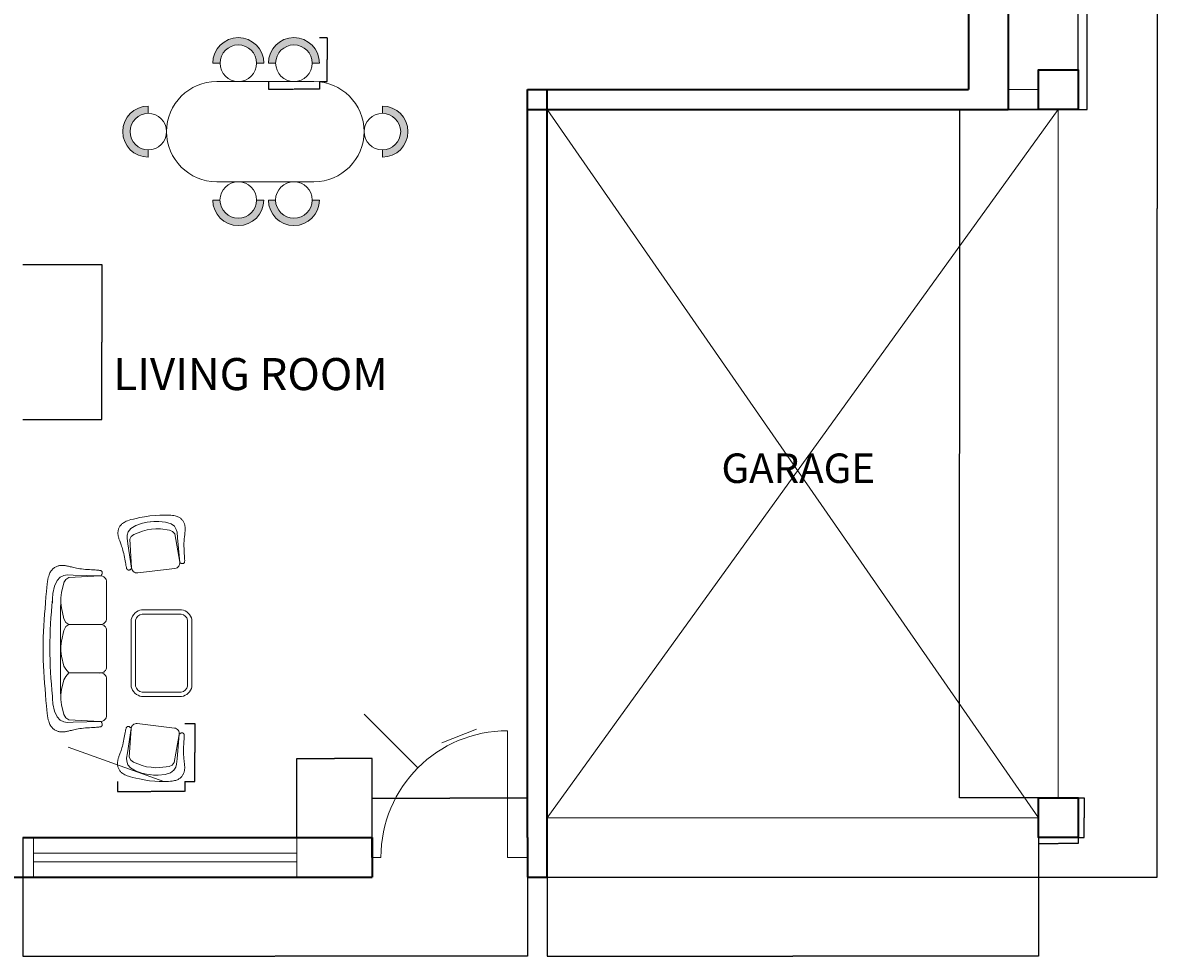
# Model space of a CAD drawing. Units: millimetres. Extents: x 2511 to 24632, y 2213 to 12972.
# Tile 2 of 5: x 6023 to 12605, y 2213 to 7630. Entities that reach past the tile are written whole.
import ezdxf

# ---------------------------------------------------------------- set-up
doc = ezdxf.new("R2010")
doc.units = ezdxf.units.MM
for name, color, linetype, lineweight in [('A-ANNO-DIMS', 2, 'Continuous', 18), ('A-AREA-IDEN', 7, 'Continuous', 20), ('A-COLS', 7, 'Continuous', 35), ('A-FLOR-GARG', 7, 'Continuous', 18), ('A-WALL', 7, 'Continuous', 35), ('doors', 50, 'Continuous', 18), ('Imaginery', 30, 'Continuous', 13), ('windows', 70, 'Continuous', 18)]:
    doc.layers.add(name, color=color, linetype=linetype, lineweight=lineweight)
doc.layers.add('A-FURN', color=11, linetype='Continuous', lineweight=18, true_color=0xf27172)
doc.layers.add('A-FURN-PATT', color=152, linetype='Continuous', lineweight=9, true_color=0x2776bb)
doc.styles.get("Standard").update_dxf_attribs({"font": 'arial.ttf'})
doc.dimstyles.get("Standard").update_dxf_attribs({"dimtxt": 0.18, "dimasz": 0.18, "dimexe": 0.18, "dimexo": 0.0625, "dimgap": 0.09, "dimtad": 0, "dimtih": 1, "dimtoh": 1, "dimdec": 4, "dimzin": 0, "dimdsep": 46, "dimtxsty": 'Standard', "dimcen": 0.09, "dimadec": 0, "dimazin": 0, "dimtfac": 1, "dimtdec": 4, "dimtofl": 0, "dimtmove": 0, "dimatfit": 3, "dimfxl": 1, "dimtolj": 1, "dimtzin": 0, "dimarcsym": 0})

# ---------------------------------------------------------------- blocks, each defined once
blk = doc.blocks.new('ARMCHAIR-PLAN')
for p, q in [((114.6, 335.8), (330.9, 309.9)), ((41.8, 265.4), (39.9, 255.1)), ((43.5, 275), (41.8, 265.4)), ((45, 283.8), (43.5, 275)), ((46.5, 291.5), (45, 283.8)), ((47.7, 297.8), (46.5, 291.5)), ((48.8, 302.8), (47.7, 297.8)), ((49.8, 306.7), (48.8, 302.8)), ((50.7, 309.7), (49.8, 306.7)), ((51.5, 311.9), (50.7, 309.7)), ((52.3, 313.6), (51.5, 311.9)), ((53.1, 314.8), (52.3, 313.6)), ((53.9, 315.7), (53.1, 314.8)), ((54.8, 316.6), (53.9, 315.7)), ((55.7, 317.3), (54.8, 316.6)), ((56.7, 317.9), (55.7, 317.3)), ((57.8, 318.4), (56.7, 317.9)), ((58.9, 318.8), (57.8, 318.4)), ((79.4, 308.1), (57.8, 166.2)), ((60.2, 319.1), (58.9, 318.8)), ((61.6, 319.2), (60.2, 319.1)), ((63.1, 319.2), (61.6, 319.2)), ((64.7, 319), (63.1, 319.2)), ((66.5, 318.7), (64.7, 319)), ((68.4, 318.1), (66.5, 318.7)), ((70.4, 317.1), (68.4, 318.1)), ((68.4, 140.6), (79.3, 306.5)), ((72.5, 315.6), (70.4, 317.1)), ((74.7, 313.7), (72.5, 315.6)), ((77, 311.3), (74.7, 313.7)), ((79.4, 308.1), (77, 311.3)), ((79.2, 305.4), (79.4, 305)), ((79.4, 305), (79.2, 305)), ((358.3, 273.1), (329.8, 109.3)), ((358.7, 274.8), (346.2, 131.7)), ((358.7, 274.8), (361.7, 277.2)), ((361.7, 277.2), (364.5, 279.1)), ((364.5, 279.1), (367.2, 280.4)), ((367.2, 280.4), (369.5, 281.3)), ((369.5, 281.3), (371.7, 281.8)), ((371.7, 281.8), (373.7, 282)), ((373.7, 282), (375.5, 281.9)), ((375.5, 281.9), (377.2, 281.7)), ((377.2, 281.7), (378.6, 281.3)), ((378.6, 281.3), (379.9, 280.8)), ((379.9, 280.8), (381.1, 280.3)), ((381.1, 280.3), (382.2, 279.6)), ((382.2, 279.6), (383.1, 278.9)), ((383.1, 278.9), (383.9, 278.1)), ((383.9, 278.1), (384.6, 277.1)), ((384.6, 277.1), (385.3, 276.1)), ((385.3, 276.1), (385.8, 275)), ((385.8, 275), (386.3, 273.7)), ((386.3, 273.7), (386.7, 271.9)), ((386.7, 271.9), (387, 269.5)), ((387, 269.5), (387.2, 266.4)), ((387.2, 266.4), (387.2, 262.3)), ((28.8, 203.9), (26.4, 195.3)), ((31.2, 213.2), (28.8, 203.9)), ((33.6, 223.3), (31.2, 213.2)), ((35.8, 233.8), (33.6, 223.3)), ((37.9, 244.5), (35.8, 233.8)), ((39.9, 255.1), (37.9, 244.5)), ((384, 203.1), (383.5, 192.2)), ((384.6, 213.9), (384, 203.1)), ((385.2, 224.3), (384.6, 213.9)), ((385.8, 234.1), (385.2, 224.3)), ((386.4, 243), (385.8, 234.1)), ((386.8, 250.8), (386.4, 243)), ((387.1, 257.2), (386.8, 250.8)), ((387.2, 262.3), (387.1, 257.2)), ((4.7, 133), (3.7, 129.1)), ((5.9, 137), (4.7, 133)), ((7.2, 141.2), (5.9, 137)), ((8.8, 145.6), (7.2, 141.2)), ((10.4, 150.4), (8.8, 145.6)), ((12.3, 155.4), (10.4, 150.4)), ((14.4, 160.9), (12.3, 155.4)), ((16.6, 166.7), (14.4, 160.9)), ((18.9, 173), (16.6, 166.7)), ((21.4, 179.9), (18.9, 173)), ((23.9, 187.3), (21.4, 179.9)), ((26.4, 195.3), (23.9, 187.3)), ((57.8, 166.2), (53.1, 134.6)), ((53.1, 134.6), (53.9, 117)), ((77.1, 124), (68.4, 140.6)), ((346.2, 131.7), (343.4, 99.9)), ((383.2, 181.5), (383.1, 171.2)), ((383.1, 171.2), (383.3, 161.5)), ((383.5, 192.2), (383.2, 181.5)), ((383.3, 161.5), (383.6, 152.5)), ((383.6, 152.5), (384.2, 144.2)), ((384.2, 144.2), (384.9, 136.4)), ((384.9, 136.4), (385.6, 129.2)), ((0.1, 107.3), (0, 103.7)), ((0, 103.7), (0.1, 100)), ((0.3, 110.9), (0.1, 107.3)), ((0.1, 100), (0.5, 96.3)), ((0.7, 114.5), (0.3, 110.9)), ((0.5, 96.3), (1.1, 92.5)), ((1.3, 118.1), (0.7, 114.5)), ((1.1, 92.5), (1.9, 88.6)), ((2, 121.7), (1.3, 118.1)), ((1.9, 88.6), (2.9, 84.6)), ((2.7, 125.4), (2, 121.7)), ((3.7, 129.1), (2.7, 125.4)), ((2.9, 84.6), (4.2, 80.6)), ((4.2, 80.6), (5.8, 76.7)), ((5.8, 76.7), (7.6, 72.7)), ((7.6, 72.7), (9.6, 68.9)), ((9.6, 68.9), (11.8, 65.1)), ((53.9, 117), (60.2, 96.8)), ((60.2, 96.8), (75.6, 78.4)), ((75.6, 78.4), (103.8, 61.4)), ((92.3, 112.4), (77.1, 124)), ((142.6, 92.8), (92.3, 112.4)), ((169.1, 85.7), (142.6, 92.8)), ((195, 82.6), (169.1, 85.7)), ((219, 79.7), (195, 82.6)), ((246.4, 80.3), (219, 79.7)), ((299.9, 87.6), (246.4, 80.3)), ((317.4, 95.2), (299.9, 87.6)), ((329.8, 109.3), (317.4, 95.2)), ((338.5, 83), (327.5, 64.8)), ((343.4, 99.9), (338.5, 83)), ((385.6, 129.2), (386.4, 122.5)), ((386.4, 122.5), (387.2, 116.3)), ((387.2, 116.3), (387.9, 110.5)), ((387.9, 110.5), (388.5, 105.2)), ((388.5, 105.2), (389, 100.2)), ((389, 100.2), (389.5, 95.5)), ((389.5, 68.1), (389.1, 64.5)), ((389.5, 95.5), (389.8, 91.1)), ((389.8, 71.7), (389.5, 68.1)), ((389.8, 91.1), (390, 86.9)), ((390, 75.4), (389.8, 71.7)), ((390, 86.9), (390.1, 82.9)), ((390.1, 79.1), (390, 75.4)), ((390.1, 82.9), (390.1, 79.1)), ((11.8, 65.1), (14.2, 61.5)), ((14.2, 61.5), (16.9, 58)), ((16.9, 58), (19.9, 54.7)), ((19.9, 54.7), (23.3, 51.5)), ((23.3, 51.5), (27.1, 48.4)), ((27.1, 48.4), (31.4, 45.4)), ((31.4, 45.4), (36.4, 42.4)), ((36.4, 42.4), (42, 39.4)), ((42, 39.4), (48.5, 36.4)), ((48.5, 36.4), (55.8, 33.3)), ((55.8, 33.3), (64.7, 30.1)), ((64.7, 30.1), (75.7, 26.7)), ((75.7, 26.7), (89.5, 23)), ((89.5, 23), (106.7, 19)), ((103.8, 61.4), (142.1, 48)), ((106.7, 19), (128, 14.5)), ((128, 14.5), (154.1, 9.5)), ((142.1, 48), (168.7, 41.9)), ((154.1, 9.5), (185.6, 3.9)), ((168.7, 41.9), (189.9, 39.4)), ((216.9, 2), (185.6, 3.9)), ((209.1, 37.1), (188, 39.6)), ((236.4, 36.7), (209.1, 37.1)), ((243, 0.7), (216.9, 2)), ((276.9, 40.7), (236.4, 36.7)), ((264.4, 0.1), (243, 0.7)), ((281.9, 0), (264.4, 0.1)), ((308.3, 50.5), (276.9, 40.7)), ((296.1, 0.3), (281.9, 0)), ((307.5, 1.1), (296.1, 0.3)), ((316.8, 2.1), (307.5, 1.1)), ((327.5, 64.8), (308.3, 50.5)), ((324.7, 3.4), (316.8, 2.1)), ((331.7, 4.8), (324.7, 3.4)), ((337.9, 6.4), (331.7, 4.8)), ((343.4, 8.1), (337.9, 6.4)), ((348.3, 10), (343.4, 8.1)), ((352.8, 12.2), (348.3, 10)), ((356.8, 14.5), (352.8, 12.2)), ((360.5, 17), (356.8, 14.5)), ((363.9, 19.7), (360.5, 17)), ((367.1, 22.6), (363.9, 19.7)), ((370.2, 25.8), (367.1, 22.6)), ((373, 29), (370.2, 25.8)), ((375.7, 32.4), (373, 29)), ((378.1, 35.9), (375.7, 32.4)), ((380.3, 39.5), (378.1, 35.9)), ((382.3, 43.1), (380.3, 39.5)), ((384, 46.7), (382.3, 43.1)), ((385.5, 50.3), (384, 46.7)), ((386.7, 53.8), (385.5, 50.3)), ((387.7, 57.4), (386.7, 53.8)), ((388.5, 60.9), (387.7, 57.4)), ((389.1, 64.5), (388.5, 60.9))]:
    blk.add_line(p, q)
for centre, start, end in [((110.8, 304.4), 83.18314, 176.2418), ((327.2, 278.5), 350.12448, 83.18314)]:
    blk.add_arc(centre, 31.6, start, end)
blk = doc.blocks.new('DINING-CHAIR-PLAN')
for p, q in [((42.1, 106.1), (0, 106.1)), ((254.4, 106.1), (296.5, 106.1))]:
    blk.add_line(p, q)
blk.add_circle((148.3, 106.1), 106.1)
blk.add_arc((148.3, 106.1), 148.3, 0, 180)
blk = doc.blocks.new('WINDOW-1528-PLAN')
for p, q in [((0, 140), (1528, 140)), ((0, 90), (1528, 90))]:
    blk.add_line(p, q)
blk.add_lwpolyline([(0, 230), (1528, 230), (1528, 0), (0, 0)], close=True)
blk = doc.blocks.new('COLUMN-230-SQUARE')
blk.add_lwpolyline([(230, 0), (0, 0), (0, 230), (230, 230), (230, 115)], close=True)
blk = doc.blocks.new('*D17')
at = {"layer": 'A-ANNO-DIMS', "color": 0, "lineweight": -2, "transparency": 16777216}
for p, q in [((7448.5, 7289), (7448.5, 7244.4)), ((7448.6, 7244.5), (7595.2, 7244.5)), ((7744.8, 7244.5), (7598.2, 7244.5)), ((7745, 7289), (7745, 7244.4))]:
    blk.add_line(p, q, dxfattribs=at)
at = {"layer": 'A-ANNO-DIMS', "color": 0, "transparency": 16777216}
for points in [[(7448.6, 7244.6), (7448.6, 7244.5), (7448.5, 7244.5)], [(7744.8, 7244.6), (7744.8, 7244.5), (7745, 7244.5)]]:
    blk.add_solid(points, dxfattribs=at)
at = {"layer": 'Defpoints', "color": 0, "transparency": 16777216}
for p in [(7448.5, 7289), (7745, 7289), (7745, 7244.5)]:
    blk.add_point(p, dxfattribs=at)
at = {"layer": 'A-ANNO-DIMS', "color": 0, "transparency": 16777216, "insert": (7596.7, 7244.5), "char_height": 0.18, "attachment_point": 5}
blk.add_mtext('\\A1;DINING CHAIR 297 TYP.', dxfattribs=at)
blk = doc.blocks.new('*D18')
at = {"layer": 'A-ANNO-DIMS', "color": 0, "lineweight": -2, "transparency": 16777216}
for p, q in [((7745, 7543.4), (7789.6, 7543.4)), ((7789.4, 7543.2), (7789.4, 7416.4)), ((7789.4, 7289.2), (7789.4, 7416)), ((7745, 7289), (7789.6, 7289))]:
    blk.add_line(p, q, dxfattribs=at)
at = {"layer": 'A-ANNO-DIMS', "color": 0, "transparency": 16777216}
for points in [[(7789.4, 7543.2), (7789.5, 7543.2), (7789.4, 7543.4)], [(7789.4, 7289.2), (7789.5, 7289.2), (7789.4, 7289)]]:
    blk.add_solid(points, dxfattribs=at)
at = {"layer": 'Defpoints', "color": 0, "transparency": 16777216}
for p in [(7745, 7543.4), (7789.4, 7543.4), (7745, 7289)]:
    blk.add_point(p, dxfattribs=at)
at = {"layer": 'A-ANNO-DIMS', "color": 0, "transparency": 16777216, "insert": (7789.4, 7416.2), "char_height": 0.18, "attachment_point": 5}
blk.add_mtext('\\A1;254 TYP.', dxfattribs=at)
blk = doc.blocks.new('*D25')
at = {"layer": 'A-ANNO-DIMS', "color": 0, "lineweight": -2, "transparency": 16777216}
for p, q in [((6572.9, 3227.2), (6572.9, 3168.6)), ((6963, 3227.2), (6963, 3168.6)), ((6573.1, 3168.8), (6766.6, 3168.8)), ((6962.8, 3168.8), (6769.3, 3168.8))]:
    blk.add_line(p, q, dxfattribs=at)
at = {"layer": 'A-ANNO-DIMS', "color": 0, "transparency": 16777216}
for points in [[(6573.1, 3168.8), (6573.1, 3168.8), (6572.9, 3168.8)], [(6962.8, 3168.8), (6962.8, 3168.8), (6963, 3168.8)]]:
    blk.add_solid(points, dxfattribs=at)
at = {"layer": 'Defpoints', "color": 0, "transparency": 16777216}
for p in [(6572.9, 3227.3), (6963, 3227.3), (6963, 3168.8)]:
    blk.add_point(p, dxfattribs=at)
at = {"layer": 'A-ANNO-DIMS', "color": 0, "transparency": 16777216, "insert": (6768, 3168.8), "char_height": 0.18, "attachment_point": 5}
blk.add_mtext('\\A1;ARMCHAIR 390 TYP.', dxfattribs=at)
blk = doc.blocks.new('*D26')
at = {"layer": 'A-ANNO-DIMS', "color": 0, "lineweight": -2, "transparency": 16777216}
for p, q in [((6963.1, 3564.1), (7021.7, 3564.1)), ((7021.5, 3563.9), (7021.5, 3395.9)), ((7021.5, 3227.5), (7021.5, 3395.5)), ((6963.1, 3227.3), (7021.7, 3227.3))]:
    blk.add_line(p, q, dxfattribs=at)
at = {"layer": 'A-ANNO-DIMS', "color": 0, "transparency": 16777216}
for points in [[(7021.5, 3563.9), (7021.6, 3563.9), (7021.5, 3564.1)], [(7021.5, 3227.5), (7021.6, 3227.5), (7021.5, 3227.3)]]:
    blk.add_solid(points, dxfattribs=at)
at = {"layer": 'Defpoints', "color": 0, "transparency": 16777216}
for p in [(6963, 3564.1), (7021.5, 3564.1), (6963, 3227.3)]:
    blk.add_point(p, dxfattribs=at)
at = {"layer": 'A-ANNO-DIMS', "color": 0, "transparency": 16777216, "insert": (7021.5, 3395.7), "char_height": 0.18, "attachment_point": 5}
blk.add_mtext('\\A1;337 TYP.', dxfattribs=at)
blk = doc.blocks.new('*D29')
at = {"layer": 'A-ANNO-DIMS', "color": 0, "lineweight": -2, "transparency": 16777216}
for p, q in [((11916.2, 2901.8), (11916.2, 2867.2)), ((12146.2, 2901.8), (12146.2, 2867.2)), ((11916.4, 2867.4), (12030, 2867.4)), ((12146, 2867.4), (12032.4, 2867.4))]:
    blk.add_line(p, q, dxfattribs=at)
at = {"layer": 'A-ANNO-DIMS', "color": 0, "transparency": 16777216}
for points in [[(11916.4, 2867.4), (11916.4, 2867.3), (11916.2, 2867.4)], [(12146, 2867.4), (12146, 2867.3), (12146.2, 2867.4)]]:
    blk.add_solid(points, dxfattribs=at)
at = {"layer": 'Defpoints', "color": 0, "transparency": 16777216}
for p in [(11916.2, 2901.9), (12146.2, 2901.9), (12146.2, 2867.4)]:
    blk.add_point(p, dxfattribs=at)
at = {"layer": 'A-ANNO-DIMS', "color": 0, "transparency": 16777216, "insert": (12031.2, 2867.4), "char_height": 0.18, "attachment_point": 5}
blk.add_mtext('\\A1;COLUMN 230 TYP.', dxfattribs=at)
blk = doc.blocks.new('*D30')
at = {"layer": 'A-ANNO-DIMS', "color": 0, "lineweight": -2, "transparency": 16777216}
for p, q in [((12146.3, 3131.9), (12180.9, 3131.9)), ((12180.7, 3131.7), (12180.7, 3017)), ((12180.7, 2902), (12180.7, 3016.7)), ((12146.3, 2901.9), (12180.9, 2901.9))]:
    blk.add_line(p, q, dxfattribs=at)
at = {"layer": 'A-ANNO-DIMS', "color": 0, "transparency": 16777216}
for points in [[(12180.7, 3131.7), (12180.7, 3131.7), (12180.7, 3131.9)], [(12180.7, 2902), (12180.7, 2902), (12180.7, 2901.9)]]:
    blk.add_solid(points, dxfattribs=at)
at = {"layer": 'Defpoints', "color": 0, "transparency": 16777216}
for p in [(12146.2, 3131.9), (12180.7, 3131.9), (12146.2, 2901.9)]:
    blk.add_point(p, dxfattribs=at)
at = {"layer": 'A-ANNO-DIMS', "color": 0, "transparency": 16777216, "insert": (12180.7, 3016.9), "char_height": 0.18, "attachment_point": 5}
blk.add_mtext('\\A1;230 TYP.', dxfattribs=at)
blk = doc.blocks.new('*D35')
at = {"layer": 'A-ANNO-DIMS', "color": 0, "lineweight": -2, "transparency": 16777216}
for p, q in [((2970.2, 10431.9), (2970.2, 10891)), ((2970.4, 10890.9), (7557.9, 10890.9)), ((12146, 10890.9), (7558.6, 10890.9)), ((12146.2, 7356.9), (12146.2, 10891))]:
    blk.add_line(p, q, dxfattribs=at)
at = {"layer": 'A-ANNO-DIMS', "color": 0, "transparency": 16777216}
for points in [[(2970.4, 10890.9), (2970.4, 10890.8), (2970.2, 10890.9)], [(12146, 10890.9), (12146, 10890.8), (12146.2, 10890.9)]]:
    blk.add_solid(points, dxfattribs=at)
at = {"layer": 'Defpoints', "color": 0, "transparency": 16777216}
for p in [(12146.2, 10890.9), (2970.2, 10431.9), (12146.2, 7356.9)]:
    blk.add_point(p, dxfattribs=at)
at = {"layer": 'A-ANNO-DIMS', "color": 0, "transparency": 16777216, "insert": (7558.2, 10890.9), "char_height": 0.18, "attachment_point": 5}
blk.add_mtext('\\A1;9176', dxfattribs=at)
blk = doc.blocks.new('*D36')
at = {"layer": 'A-ANNO-DIMS', "color": 0, "lineweight": -2, "transparency": 16777216}
for p, q in [((11740.3, 10431.9), (12605.4, 10431.9)), ((12605.2, 10431.7), (12605.2, 6552)), ((12605.2, 2672), (12605.2, 6551.7)), ((9066.3, 2671.9), (12605.4, 2671.9))]:
    blk.add_line(p, q, dxfattribs=at)
at = {"layer": 'A-ANNO-DIMS', "color": 0, "transparency": 16777216}
for points in [[(12605.2, 10431.7), (12605.2, 10431.7), (12605.2, 10431.9)], [(12605.2, 2672), (12605.2, 2672), (12605.2, 2671.9)]]:
    blk.add_solid(points, dxfattribs=at)
at = {"layer": 'Defpoints', "color": 0, "transparency": 16777216}
for p in [(11740.2, 10431.9), (12605.2, 10431.9), (9066.2, 2671.9)]:
    blk.add_point(p, dxfattribs=at)
at = {"layer": 'A-ANNO-DIMS', "color": 0, "transparency": 16777216, "insert": (12605.2, 6551.9), "char_height": 0.18, "attachment_point": 5}
blk.add_mtext('\\A1;7760', dxfattribs=at)
blk = doc.blocks.new('*D38')
at = {"layer": 'A-ANNO-DIMS', "color": 0, "lineweight": -2, "transparency": 16777216}
for p, q in [((6023.2, 2901.8), (6023.2, 2212.7)), ((8951.2, 2786.8), (8951.2, 2212.7)), ((6023.4, 2212.9), (7486.9, 2212.9)), ((8951, 2212.9), (7487.6, 2212.9))]:
    blk.add_line(p, q, dxfattribs=at)
at = {"layer": 'A-ANNO-DIMS', "color": 0, "transparency": 16777216}
for points in [[(6023.4, 2212.9), (6023.4, 2212.8), (6023.2, 2212.9)], [(8951, 2212.9), (8951, 2212.8), (8951.2, 2212.9)]]:
    blk.add_solid(points, dxfattribs=at)
at = {"layer": 'Defpoints', "color": 0, "transparency": 16777216}
for p in [(6023.2, 2901.9), (8951.2, 2786.9), (8951.2, 2212.9)]:
    blk.add_point(p, dxfattribs=at)
at = {"layer": 'A-ANNO-DIMS', "color": 0, "transparency": 16777216, "insert": (7487.2, 2212.9), "char_height": 0.18, "attachment_point": 5}
blk.add_mtext('\\A1;2928', dxfattribs=at)
blk = doc.blocks.new('*D39')
at = {"layer": 'A-ANNO-DIMS', "color": 0, "lineweight": -2, "transparency": 16777216}
for p, q in [((9066.214664, 3016.80126), (9066.214664, 2212.68376)), ((11916.214664, 3016.80126), (11916.214664, 2212.68376)), ((9066.394664, 2212.86376), (10490.854664, 2212.86376)), ((11916.034664, 2212.86376), (10491.574664, 2212.86376))]:
    blk.add_line(p, q, dxfattribs=at)
at = {"layer": 'A-ANNO-DIMS', "color": 0, "transparency": 16777216}
for points in [[(9066.394664, 2212.89376), (9066.394664, 2212.83376), (9066.214664, 2212.86376)], [(11916.034664, 2212.89376), (11916.034664, 2212.83376), (11916.214664, 2212.86376)]]:
    blk.add_solid(points, dxfattribs=at)
at = {"layer": 'Defpoints', "color": 0, "transparency": 16777216}
for p in [(9066.214664, 3016.86376), (11916.214664, 3016.86376), (11916.214664, 2212.86376)]:
    blk.add_point(p, dxfattribs=at)
at = {"layer": 'A-ANNO-DIMS', "color": 0, "transparency": 16777216, "insert": (10491.214664, 2212.86376), "char_height": 0.18, "attachment_point": 5}
blk.add_mtext('\\A1;2850', dxfattribs=at)
blk = doc.blocks.new('*D58')
at = {"layer": 'A-ANNO-DIMS', "color": 0, "lineweight": -2, "transparency": 16777216}
for p, q in [((11916.2, 7126.9), (11457, 7126.9)), ((11457.2, 7126.7), (11457.2, 5129.5)), ((11457.2, 3132), (11457.2, 5129.2)), ((11916.2, 3131.9), (11457, 3131.9))]:
    blk.add_line(p, q, dxfattribs=at)
at = {"layer": 'A-ANNO-DIMS', "color": 0, "transparency": 16777216}
for points in [[(11457.2, 7126.7), (11457.2, 7126.7), (11457.2, 7126.9)], [(11457.2, 3132), (11457.2, 3132), (11457.2, 3131.9)]]:
    blk.add_solid(points, dxfattribs=at)
at = {"layer": 'Defpoints', "color": 0, "transparency": 16777216}
for p in [(11457.2, 7126.9), (11916.2, 7126.9), (11916.2, 3131.9)]:
    blk.add_point(p, dxfattribs=at)
at = {"layer": 'A-ANNO-DIMS', "color": 0, "transparency": 16777216, "insert": (11457.2, 5129.4), "char_height": 0.18, "attachment_point": 5}
blk.add_mtext('\\A1;3995', dxfattribs=at)
blk = doc.blocks.new('*D59')
at = {"layer": 'A-ANNO-DIMS', "color": 0, "lineweight": -2, "transparency": 16777216}
for p, q in [((11740.3, 10431.9), (12199.4, 10431.9)), ((12199.2, 10431.7), (12199.2, 8779.5)), ((12199.2, 7127), (12199.2, 8779.2)), ((11740.3, 7126.9), (12199.4, 7126.9))]:
    blk.add_line(p, q, dxfattribs=at)
at = {"layer": 'A-ANNO-DIMS', "color": 0, "transparency": 16777216}
for points in [[(12199.2, 10431.7), (12199.2, 10431.7), (12199.2, 10431.9)], [(12199.2, 7127), (12199.2, 7127), (12199.2, 7126.9)]]:
    blk.add_solid(points, dxfattribs=at)
at = {"layer": 'Defpoints', "color": 0, "transparency": 16777216}
for p in [(11740.2, 10431.9), (11740.2, 7126.9), (12199.2, 7126.9)]:
    blk.add_point(p, dxfattribs=at)
at = {"layer": 'A-ANNO-DIMS', "color": 0, "transparency": 16777216, "insert": (12199.2, 8779.4), "char_height": 0.18, "attachment_point": 5}
blk.add_mtext('\\A1;3305', dxfattribs=at)
blk = doc.blocks.new('*D60')
at = {"layer": 'A-ANNO-DIMS', "color": 0, "lineweight": -2, "transparency": 16777216}
for p, q in [((7613.2, 2901.9), (7613.2, 3361)), ((7613.4, 3360.9), (7831.9, 3360.9)), ((8051, 3360.9), (7832.5, 3360.9)), ((8051.2, 2901.9), (8051.2, 3361))]:
    blk.add_line(p, q, dxfattribs=at)
at = {"layer": 'A-ANNO-DIMS', "color": 0, "transparency": 16777216}
for points in [[(7613.4, 3360.9), (7613.4, 3360.8), (7613.2, 3360.9)], [(8051, 3360.9), (8051, 3360.8), (8051.2, 3360.9)]]:
    blk.add_solid(points, dxfattribs=at)
at = {"layer": 'Defpoints', "color": 0, "transparency": 16777216}
for p in [(8051.2, 3360.9), (7613.2, 2901.9), (8051.2, 2901.9)]:
    blk.add_point(p, dxfattribs=at)
at = {"layer": 'A-ANNO-DIMS', "color": 0, "transparency": 16777216, "insert": (7832.2, 3360.9), "char_height": 0.18, "attachment_point": 5}
blk.add_mtext('\\A1;438', dxfattribs=at)
blk = doc.blocks.new('*D61')
at = {"layer": 'A-ANNO-DIMS', "color": 0, "lineweight": -2, "transparency": 16777216}
for p, q in [((8051.2, 2671.9), (8051.2, 3131)), ((8051.4, 3130.9), (8500.9, 3130.9)), ((8951, 3130.9), (8501.5, 3130.9)), ((8951.2, 2671.9), (8951.2, 3131))]:
    blk.add_line(p, q, dxfattribs=at)
at = {"layer": 'A-ANNO-DIMS', "color": 0, "transparency": 16777216}
for points in [[(8051.4, 3130.9), (8051.4, 3130.8), (8051.2, 3130.9)], [(8951, 3130.9), (8951, 3130.8), (8951.2, 3130.9)]]:
    blk.add_solid(points, dxfattribs=at)
at = {"layer": 'Defpoints', "color": 0, "transparency": 16777216}
for p in [(8951.2, 3130.9), (8051.2, 2671.9), (8951.2, 2671.9)]:
    blk.add_point(p, dxfattribs=at)
at = {"layer": 'A-ANNO-DIMS', "color": 0, "transparency": 16777216, "insert": (8501.2, 3130.9), "char_height": 0.18, "attachment_point": 5}
blk.add_mtext('\\A1;900', dxfattribs=at)
blk = doc.blocks.new('*D62')
at = {"layer": 'A-ANNO-DIMS', "color": 0, "lineweight": -2, "transparency": 16777216}
for p, q in [((6023.3, 6226.9), (6482.4, 6226.9)), ((6482.2, 6226.7), (6482.2, 5777)), ((6482.2, 5327), (6482.2, 5776.7)), ((6023.3, 5326.9), (6482.4, 5326.9))]:
    blk.add_line(p, q, dxfattribs=at)
at = {"layer": 'A-ANNO-DIMS', "color": 0, "transparency": 16777216}
for points in [[(6482.2, 6226.7), (6482.2, 6226.7), (6482.2, 6226.9)], [(6482.2, 5327), (6482.2, 5327), (6482.2, 5326.9)]]:
    blk.add_solid(points, dxfattribs=at)
at = {"layer": 'Defpoints', "color": 0, "transparency": 16777216}
for p in [(6023.2, 6226.9), (6023.2, 5326.9), (6482.2, 5326.9)]:
    blk.add_point(p, dxfattribs=at)
at = {"layer": 'A-ANNO-DIMS', "color": 0, "transparency": 16777216, "insert": (6482.2, 5776.9), "char_height": 0.18, "attachment_point": 5}
blk.add_mtext('\\A1;900', dxfattribs=at)
blk = doc.blocks.new('*D99')
at = {"layer": 'A-ANNO-DIMS', "color": 0, "lineweight": -2, "transparency": 16777216}
for p, q in [((8004.5, 3618.4), (8004.7, 3618.4)), ((8004.7, 3618.4), (8316.4, 3306.7)), ((8836.1, 2786.9), (8836.3, 2786.9)), ((8836.2, 2786.8), (8836.2, 2787))]:
    blk.add_line(p, q, dxfattribs=at)
at = {"layer": 'A-ANNO-DIMS', "color": 0, "transparency": 16777216}
blk.add_solid([(8316.4, 3306.7), (8316.3, 3306.7), (8316.5, 3306.6)], dxfattribs=at)
at = {"layer": 'Defpoints', "color": 0, "transparency": 16777216}
for p in [(8316.5, 3306.6), (8836.2, 2786.9)]:
    blk.add_point(p, dxfattribs=at)
at = {"layer": 'A-ANNO-DIMS', "color": 0, "transparency": 16777216, "insert": (8004.1, 3618.4), "char_height": 0.18, "attachment_point": 5}
blk.add_mtext('\\A1;R735', dxfattribs=at)

msp = doc.modelspace()

# ---------------------------------------------------------------- hatches: boundary and pattern name
at = {"layer": 'A-FURN-PATT'}
h = msp.add_hatch(color=256, dxfattribs=at)
h.dxf.hatch_style = 1
h.paths.add_polyline_path([(7125.707, 7395.151), (7167.831, 7395.151, -1), (7380.088, 7395.151), (7422.212, 7395.151, 1)])
h.paths.add_polyline_path([(7448.458, 7395.151), (7490.582, 7395.151, -1), (7702.839, 7395.151), (7744.962, 7395.151, 1)])
h.paths.add_polyline_path([(6645.685, 6998.173, -0.41421356), (6751.814, 7104.302), (6751.814, 7146.426, 1), (6751.814, 6849.921), (6751.814, 6892.045, -0.41421356)])
h.paths.add_polyline_path([(8109.913, 7146.426), (8109.913, 7104.302, -0.41421356), (8216.042, 6998.173, -0.41421356), (8109.913, 6892.045), (8109.913, 6849.921, 1)])
h.paths.add_polyline_path([(7422.212, 6601.196), (7380.088, 6601.196, -1), (7167.831, 6601.196), (7125.707, 6601.196, 1)])
h.paths.add_polyline_path([(7744.962, 6601.196), (7702.839, 6601.196, -1), (7490.582, 6601.196), (7448.458, 6601.196, 1)])

# ---------------------------------------------------------------- linework, layer by layer
at = {"layer": 'A-FLOR-GARG'}
for p, q in [((11916.215, 7241.864), (11740.215, 7241.864)), ((12031.215, 7126.864), (9066.215, 3016.864)), ((9066.215, 7126.864), (11916.215, 3016.864)), ((12031.215, 7126.864), (12031.215, 3131.864)), ((11916.215, 3016.864), (9066.215, 3016.864))]:
    msp.add_line(p, q, dxfattribs=at)
at = {"layer": 'A-FURN'}
for p, q in [((7148.791, 7289.022), (7712.936, 7289.022)), ((7148.791, 6707.325), (7712.936, 6707.325)), ((6224.853, 4476.163), (6220.671, 4474.483)), ((6229.004, 4477.567), (6224.853, 4476.163)), ((6233.096, 4478.694), (6229.004, 4477.567)), ((6237.137, 4479.558), (6233.096, 4478.694)), ((6241.14, 4480.181), (6237.137, 4479.558)), ((6245.121, 4480.584), (6241.14, 4480.181)), ((6249.093, 4480.787), (6245.121, 4480.584)), ((6253.071, 4480.812), (6249.093, 4480.787)), ((6257.07, 4480.678), (6253.071, 4480.812)), ((6261.105, 4480.407), (6257.07, 4480.678)), ((6265.194, 4480.015), (6261.105, 4480.407)), ((6269.382, 4479.5), (6265.194, 4480.015)), ((6273.715, 4478.856), (6269.382, 4479.5)), ((6278.241, 4478.077), (6273.715, 4478.856)), ((6283.009, 4477.157), (6278.241, 4478.077)), ((6288.065, 4476.089), (6283.009, 4477.157)), ((6293.458, 4474.867), (6288.065, 4476.089)), ((6173.936, 4418.468), (6171.537, 4410.029)), ((6176.395, 4425.87), (6173.936, 4418.468)), ((6178.933, 4432.43), (6176.395, 4425.87)), ((6181.569, 4438.237), (6178.933, 4432.43)), ((6184.322, 4443.381), (6181.569, 4438.237)), ((6187.212, 4447.951), (6184.322, 4443.381)), ((6190.259, 4452.036), (6187.212, 4447.951)), ((6193.483, 4455.726), (6190.259, 4452.036)), ((6196.903, 4459.11), (6193.483, 4455.726)), ((6200.53, 4462.261), (6196.903, 4459.11)), ((6204.338, 4465.188), (6200.53, 4462.261)), ((6208.291, 4467.882), (6204.338, 4465.188)), ((6212.355, 4470.335), (6208.291, 4467.882)), ((6216.493, 4472.538), (6212.355, 4470.335)), ((6220.671, 4474.483), (6216.493, 4472.538)), ((6241.418, 4413.499), (6223.328, 4394.332)), ((6262.701, 4423.083), (6241.418, 4413.499)), ((6281.855, 4426.277), (6262.701, 4423.083)), ((6273.342, 4399.19), (6290.368, 4410.903)), ((6273.342, 4399.19), (6290.368, 4410.903)), ((6316.971, 4425.212), (6281.855, 4426.277)), ((6290.368, 4410.903), (6472.945, 4420.659)), ((6299.235, 4473.485), (6293.458, 4474.867)), ((6305.445, 4471.945), (6299.235, 4473.485)), ((6312.132, 4470.285), (6305.445, 4471.945)), ((6319.343, 4468.55), (6312.132, 4470.285)), ((6474.801, 4420.11), (6316.971, 4425.212)), ((6327.124, 4466.786), (6319.343, 4468.55)), ((6335.52, 4465.038), (6327.124, 4466.786)), ((6344.577, 4463.352), (6335.52, 4465.038)), ((6354.34, 4461.775), (6344.577, 4463.352)), ((6364.856, 4460.352), (6354.34, 4461.775)), ((6376.113, 4459.117), (6364.856, 4460.352)), ((6387.87, 4458.056), (6376.113, 4459.117)), ((6399.832, 4457.145), (6387.87, 4458.056)), ((6411.699, 4456.359), (6399.832, 4457.145)), ((6423.176, 4455.673), (6411.699, 4456.359)), ((6433.965, 4455.061), (6423.176, 4455.673)), ((6443.769, 4454.5), (6433.965, 4455.061)), ((6452.291, 4453.963), (6443.769, 4454.5)), ((6459.313, 4453.429), (6452.291, 4453.963)), ((6464.941, 4452.887), (6459.313, 4453.429)), ((6469.359, 4452.328), (6464.941, 4452.887)), ((6472.753, 4451.745), (6469.359, 4452.328)), ((6471.775, 4419.998), (6471.365, 4419.761)), ((6471.365, 4419.761), (6471.365, 4419.976)), ((6475.307, 4451.128), (6472.753, 4451.745)), ((6474.801, 4420.11), (6477.894, 4423.132)), ((6477.206, 4450.469), (6475.307, 4451.128)), ((6478.636, 4449.76), (6477.206, 4450.469)), ((6477.894, 4423.132), (6480.301, 4425.977)), ((6479.781, 4448.994), (6478.636, 4449.76)), ((6480.794, 4448.16), (6479.781, 4448.994)), ((6480.301, 4425.977), (6482.1, 4428.646)), ((6481.704, 4447.247), (6480.794, 4448.16)), ((6482.505, 4446.242), (6481.704, 4447.247)), ((6482.1, 4428.646), (6483.37, 4431.141)), ((6483.195, 4445.134), (6482.505, 4446.242)), ((6483.768, 4443.909), (6483.195, 4445.134)), ((6483.37, 4431.141), (6484.191, 4433.463)), ((6484.22, 4442.555), (6483.768, 4443.909)), ((6484.191, 4433.463), (6484.641, 4435.614)), ((6484.548, 4441.059), (6484.22, 4442.555)), ((6484.747, 4439.41), (6484.548, 4441.059)), ((6484.641, 4435.614), (6484.8, 4437.596)), ((6484.8, 4437.596), (6484.747, 4439.41)), ((6162.515, 4352.564), (6160.399, 4328.672)), ((6164.685, 4371.926), (6162.515, 4352.564)), ((6166.913, 4387.477), (6164.685, 4371.926)), ((6169.196, 4399.939), (6166.913, 4387.477)), ((6171.537, 4410.029), (6169.196, 4399.939)), ((6208.431, 4361.322), (6198.854, 4317.663)), ((6223.328, 4394.332), (6208.431, 4361.322)), ((6262.701, 4381.088), (6273.342, 4399.19)), ((6158.339, 4299.531), (6156.333, 4264.421)), ((6160.399, 4328.672), (6158.339, 4299.531)), ((6198.854, 4317.663), (6195.661, 4287.847)), ((6195.661, 4287.847), (6195.661, 4264.421)), ((6195.661, 4277.287), (6195.661, 4266.469)), ((6247.803, 4041.509), (6262.701, 4103.052)), ((6262.701, 4103.052), (6273.342, 4126.139)), ((6509.576, 4103.856), (6509.576, 3891.83)), ((6243.547, 4011.693), (6247.803, 4041.509)), ((6243.547, 4010.614), (6243.547, 4011.693)), ((6243.547, 3983.993), (6243.547, 4010.614)), ((6247.803, 3954.177), (6243.547, 3983.993)), ((6262.701, 3896.676), (6247.803, 3954.177)), ((6262.701, 3896.077), (6273.342, 3877.974)), ((6262.701, 3817.533), (6273.342, 3835.635)), ((6273.342, 3877.974), (6290.368, 3857.834)), ((6273.342, 3835.635), (6290.368, 3857.834)), ((6290.368, 3857.834), (6472.945, 3857.104)), ((6290.368, 3857.834), (6472.945, 3857.104)), ((6471.775, 3857.042), (6471.365, 3856.805)), ((6471.365, 3856.805), (6471.365, 3857.02)), ((6471.775, 3856.568), (6471.365, 3856.805)), ((6471.365, 3856.805), (6471.365, 3856.59)), ((6509.576, 3610.352), (6509.576, 3822.378)), ((6247.803, 3760.031), (6243.547, 3730.215)), ((6262.701, 3817.533), (6247.803, 3760.031)), ((6158.339, 3696.156), (6156.333, 3731.266)), ((6160.399, 3667.015), (6158.339, 3696.156)), ((6195.661, 3707.839), (6195.661, 3721.6)), ((6198.854, 3678.024), (6195.661, 3707.839)), ((6243.547, 3731.266), (6243.547, 3702.515)), ((6243.547, 3730.215), (6243.547, 3731.266)), ((6243.547, 3702.515), (6247.803, 3672.699)), ((6162.515, 3643.123), (6160.399, 3667.015)), ((6164.685, 3623.761), (6162.515, 3643.123)), ((6166.913, 3608.209), (6164.685, 3623.761)), ((6208.431, 3634.365), (6198.854, 3678.024)), ((6223.328, 3601.355), (6208.431, 3634.365)), ((6247.803, 3672.699), (6262.701, 3615.198)), ((6169.196, 3595.748), (6166.913, 3608.209)), ((6171.537, 3585.657), (6169.196, 3595.748)), ((6173.936, 3577.218), (6171.537, 3585.657)), ((6176.395, 3569.816), (6173.936, 3577.218)), ((6178.933, 3563.256), (6176.395, 3569.816)), ((6181.569, 3557.449), (6178.933, 3563.256)), ((6184.322, 3552.305), (6181.569, 3557.449)), ((6241.418, 3582.188), (6223.328, 3601.355)), ((6262.701, 3572.604), (6241.418, 3582.188)), ((6262.701, 3615.198), (6273.342, 3597.095)), ((6281.855, 3569.409), (6262.701, 3572.604)), ((6273.342, 3597.095), (6290.368, 3585.382)), ((6316.971, 3570.474), (6281.855, 3569.409)), ((6290.368, 3585.382), (6472.945, 3575.626)), ((6474.801, 3575.577), (6316.971, 3570.474)), ((6471.365, 3575.926), (6471.365, 3575.711)), ((6471.775, 3575.689), (6471.365, 3575.926)), ((6474.801, 3575.577), (6477.894, 3572.554)), ((6477.894, 3572.554), (6480.301, 3569.71)), ((6480.301, 3569.71), (6482.1, 3567.04)), ((6482.1, 3567.04), (6483.37, 3564.546)), ((6483.37, 3564.546), (6484.191, 3562.223)), ((6484.191, 3562.223), (6484.641, 3560.072)), ((6484.548, 3554.627), (6484.22, 3553.132)), ((6484.747, 3556.276), (6484.548, 3554.627)), ((6484.641, 3560.072), (6484.8, 3558.09)), ((6484.8, 3558.09), (6484.747, 3556.276)), ((6187.212, 3547.736), (6184.322, 3552.305)), ((6190.259, 3543.651), (6187.212, 3547.736)), ((6193.483, 3539.961), (6190.259, 3543.651)), ((6196.903, 3536.577), (6193.483, 3539.961)), ((6200.53, 3533.425), (6196.903, 3536.577)), ((6204.338, 3530.498), (6200.53, 3533.425)), ((6208.291, 3527.804), (6204.338, 3530.498)), ((6212.355, 3525.351), (6208.291, 3527.804)), ((6216.493, 3523.148), (6212.355, 3525.351)), ((6220.671, 3521.203), (6216.493, 3523.148)), ((6224.853, 3519.524), (6220.671, 3521.203)), ((6229.004, 3518.119), (6224.853, 3519.524)), ((6233.096, 3516.993), (6229.004, 3518.119)), ((6237.137, 3516.128), (6233.096, 3516.993)), ((6241.14, 3515.505), (6237.137, 3516.128)), ((6245.121, 3515.102), (6241.14, 3515.505)), ((6249.093, 3514.899), (6245.121, 3515.102)), ((6253.071, 3514.875), (6249.093, 3514.899)), ((6257.07, 3515.009), (6253.071, 3514.875)), ((6261.105, 3515.28), (6257.07, 3515.009)), ((6265.194, 3515.672), (6261.105, 3515.28)), ((6269.382, 3516.187), (6265.194, 3515.672)), ((6273.715, 3516.83), (6269.382, 3516.187)), ((6278.241, 3517.609), (6273.715, 3516.83)), ((6283.009, 3518.529), (6278.241, 3517.609)), ((6288.065, 3519.597), (6283.009, 3518.529)), ((6293.458, 3520.819), (6288.065, 3519.597)), ((6299.235, 3522.201), (6293.458, 3520.819)), ((6305.445, 3523.741), (6299.235, 3522.201)), ((6312.132, 3525.401), (6305.445, 3523.741)), ((6319.343, 3527.137), (6312.132, 3525.401)), ((6327.124, 3528.901), (6319.343, 3527.137)), ((6335.52, 3530.649), (6327.124, 3528.901)), ((6344.577, 3532.334), (6335.52, 3530.649)), ((6354.34, 3533.911), (6344.577, 3532.334)), ((6364.856, 3535.334), (6354.34, 3533.911)), ((6376.113, 3536.57), (6364.856, 3535.334)), ((6387.87, 3537.63), (6376.113, 3536.57)), ((6399.832, 3538.541), (6387.87, 3537.63)), ((6411.699, 3539.328), (6399.832, 3538.541)), ((6423.176, 3540.014), (6411.699, 3539.328)), ((6433.965, 3540.625), (6423.176, 3540.014)), ((6443.769, 3541.187), (6433.965, 3540.625)), ((6452.291, 3541.723), (6443.769, 3541.187)), ((6459.313, 3542.257), (6452.291, 3541.723)), ((6464.941, 3542.799), (6459.313, 3542.257)), ((6469.359, 3543.358), (6464.941, 3542.799)), ((6472.753, 3543.942), (6469.359, 3543.358)), ((6475.307, 3544.559), (6472.753, 3543.942)), ((6477.206, 3545.217), (6475.307, 3544.559)), ((6478.636, 3545.926), (6477.206, 3545.217)), ((6479.781, 3546.693), (6478.636, 3545.926)), ((6480.794, 3547.527), (6479.781, 3546.693)), ((6481.704, 3548.44), (6480.794, 3547.527)), ((6482.505, 3549.444), (6481.704, 3548.44)), ((6483.195, 3550.553), (6482.505, 3549.444)), ((6483.768, 3551.778), (6483.195, 3550.553)), ((6484.22, 3553.132), (6483.768, 3551.778))]:
    msp.add_line(p, q, dxfattribs=at)
for points in [[(6472.945, 4138.582), (6290.368, 4137.852), (6472.945, 4138.582, 0.42993712), (6509.576, 4173.308), (6509.576, 4385.334, 0.42993712), (6472.945, 4420.06)], [(6195.661, 3721.6, -0.05093597), (6195.661, 4282.427, 12.16734757)], [(6156.333, 3731.266, -0.05357962), (6156.333, 4264.421, 12.16376721)], [(6243.547, 4266.55, 0.00498852), (6243.547, 3716.89, 0.84700309)]]:
    msp.add_lwpolyline(points, format="xyb", dxfattribs=at)
msp.add_lwpolyline([(6262.701, 4380.489), (6247.803, 4322.987), (6243.547, 4293.172), (6243.547, 4266.55), (6243.547, 4265.471), (6247.803, 4235.655), (6262.701, 4171.081), (6273.342, 4149.566), (6290.368, 4137.852), (6273.342, 4126.139)], dxfattribs=at)
for points in [[(7005.288, 4166.604), (7005.288, 3777.087, -0.30454236), (6945.011, 3720.287), (6713.399, 3720.287, -0.30454236), (6653.122, 3777.087), (6653.122, 4166.604, -0.30454236), (6713.399, 4223.404), (6945.011, 4223.404, -0.30454236)], [(6980.132, 4163.481), (6980.132, 3780.21, -0.28023346), (6942.722, 3745.443), (6715.688, 3745.443, -0.28023346), (6678.278, 3780.21), (6678.278, 4163.481, -0.28023346), (6715.688, 4198.248), (6942.722, 4198.248, -0.28023346)]]:
    msp.add_lwpolyline(points, format="xyb", close=True, dxfattribs=at)
for centre, radius, start, end in [((7148.791, 6998.173), 290.849, 90, 270), ((7712.936, 6998.173), 290.849, 270, 90), ((6474.801, 4103.856), 34.775, 0, 93.0586561), ((6474.801, 3891.83), 34.775, 266.9413439, 0), ((6474.801, 3891.83), 34.775, 266.9413439, 0), ((6474.801, 3822.378), 34.775, 0, 93.0586561), ((6474.801, 3822.378), 34.775, 0, 93.0586561), ((6474.801, 3822.378), 34.775, 0, 93.0586561), ((6474.801, 3610.352), 34.775, 266.9413439, 0)]:
    msp.add_arc(centre, radius, start, end, dxfattribs=at)
at = {"layer": 'A-WALL'}
for p, q in [((11740.215, 10431.864), (11740.215, 7126.864)), ((11510.215, 10201.864), (11510.215, 7241.864)), ((8951.215, 2901.864), (8951.215, 7241.864)), ((8951.215, 7241.864), (11510.215, 7241.864)), ((9066.215, 2671.864), (9066.215, 7241.864)), ((8951.215, 7126.864), (11740.215, 7126.864)), ((6023.215, 2901.864), (8051.215, 2901.864)), ((8051.215, 2786.864), (8051.215, 2901.864)), ((8051.215, 2901.864), (8051.215, 2671.864)), ((8951.215, 2901.864), (8951.215, 2671.864)), ((2970.215, 2671.864), (8051.215, 2671.864)), ((8951.215, 2671.864), (9066.215, 2671.864))]:
    msp.add_line(p, q, dxfattribs=at)
at = {"layer": 'doors'}
for p, q in [((8836.215, 3521.864), (8836.215, 2786.864)), ((8101.215, 2786.864), (8051.215, 2786.864)), ((8901.215, 2786.864), (8836.215, 2786.864)), ((8951.215, 2786.864), (8901.215, 2786.864))]:
    msp.add_line(p, q, dxfattribs=at)
msp.add_arc((8836.215, 2786.864), 735, 90, 180, dxfattribs=at)
at = {"layer": 'Imaginery'}
for p, q in [((8656.702, 3530.68), (8454.838, 3450.752)), ((6287.014, 3425.354), (6841.982, 3227.375))]:
    msp.add_line(p, q, dxfattribs=at)

# ---------------------------------------------------------------- block references
at = {"layer": 'A-COLS'}
for p in [(11916.215, 7126.864), (11916.215, 2901.864)]:
    msp.add_blockref('COLUMN-230-SQUARE', p, dxfattribs=at)
at = {"layer": 'A-FURN'}
for name, p in [('DINING-CHAIR-PLAN', (7125.707, 7289.022)), ('DINING-CHAIR-PLAN', (7448.458, 7289.022)), ('ARMCHAIR-PLAN', (6572.897, 3227.299))]:
    msp.add_blockref(name, p, dxfattribs=at)
for p, rotation in [((6857.942, 6849.921), 90), ((8003.784, 7146.426), 270), ((7422.212, 6707.325), 180), ((7744.962, 6707.325), 180)]:
    msp.add_blockref('DINING-CHAIR-PLAN', p, dxfattribs=dict(at, rotation=rotation))
at = {"layer": 'A-FURN', "extrusion": (0, 0, -1), "zscale": -1, "rotation": 180}
msp.add_blockref('ARMCHAIR-PLAN', (-6575.701, 4773.122), dxfattribs=at)
at = {"layer": 'windows'}
msp.add_blockref('WINDOW-1528-PLAN', (6085.224, 2671.864), dxfattribs=at)

# ---------------------------------------------------------------- texts
at = {"layer": 'A-AREA-IDEN', "attachment_point": 1}
for s, width, gutter_width, insert, char_height in [('{\\fArial|b1|i0|c0|p34;LIVING ROOM}', 1890.58512, 930.732, (6549.336, 5684.178), 186.14639), ('{\\fArial|b1|i0|c0|p34;GARAGE}', 1076.56412, 855.546, (10076.786, 5130.483), 171.10917)]:
    msp.add_mtext_dynamic_manual_height_columns(s, width=width, gutter_width=gutter_width, heights=[0], dxfattribs=dict(at, insert=insert, char_height=char_height))

# ---------------------------------------------------------------- dimensions: what is measured, and where the dimension line sits
at = {"layer": 'A-ANNO-DIMS'}
for base, p1, p2, picture, middle in [((12146.215, 10890.864), (2970.215, 10431.864), (12146.215, 7356.864), '*D35', (7558.215, 10890.864)), ((11916.215, 2212.864), (9066.215, 3016.864), (11916.215, 3016.864), '*D39', (10491.215, 2212.864)), ((8951.215, 2212.864), (6023.215, 2901.864), (8951.215, 2786.864), '*D38', (7487.215, 2212.864))]:
    dim = msp.add_linear_dim(base=base, p1=p1, p2=p2, dimstyle='Standard', override={"dimdec": 0, "dimlfac": 1, "dimrnd": 0, "dimzin": 0, "dimdsep": 46, "dimlunit": 2}, dxfattribs=at)
    dim.commit()
    dim.dimension.update_dxf_attribs({"geometry": picture, "text_midpoint": middle})
for base, p1, p2, angle, picture, middle in [((12605.215, 10431.864), (9066.215, 2671.864), (11740.215, 10431.864), 90, '*D36', (12605.215, 6551.864)), ((12199.215, 7126.864), (11740.215, 10431.864), (11740.215, 7126.864), 270, '*D59', (12199.215, 8779.364)), ((11457.215, 7126.864), (11916.215, 3131.864), (11916.215, 7126.864), 90, '*D58', (11457.215, 5129.364)), ((6482.215, 5326.864), (6023.215, 6226.864), (6023.215, 5326.864), 270, '*D62', (6482.215, 5776.864)), ((8051.215, 3360.864), (7613.212, 2901.864), (8051.215, 2901.864), 0, '*D60', (7832.213, 3360.864)), ((8951.215, 3130.864), (8051.215, 2671.864), (8951.215, 2671.864), 0, '*D61', (8501.215, 3130.864))]:
    dim = msp.add_linear_dim(base=base, p1=p1, p2=p2, angle=angle, dimstyle='Standard', override={"dimdec": 0, "dimlfac": 1, "dimrnd": 0, "dimzin": 0, "dimdsep": 46, "dimlunit": 2}, dxfattribs=at)
    dim.commit()
    dim.dimension.update_dxf_attribs({"geometry": picture, "text_midpoint": middle})
for base, p1, p2, picture, middle in [((7789.438, 7543.403), (7744.962, 7289.022), (7744.962, 7543.403), '*D18', (7789.438, 7416.212)), ((7021.53, 3564.103), (6963.012, 3227.299), (6963.012, 3564.103), '*D26', (7021.53, 3395.701)), ((12180.715, 3131.864), (12146.215, 2901.864), (12146.215, 3131.864), '*D30', (12180.715, 3016.864))]:
    dim = msp.add_linear_dim(base=base, p1=p1, p2=p2, angle=90, text='<> TYP.', dimstyle='Standard', override={"dimdec": 0, "dimlfac": 1, "dimrnd": 0, "dimzin": 0, "dimdsep": 46, "dimlunit": 2}, dxfattribs=at)
    dim.commit()
    dim.dimension.update_dxf_attribs({"geometry": picture, "text_midpoint": middle})
for base, p1, p2, text, picture, middle in [((7744.962, 7244.546), (7448.458, 7289.022), (7744.962, 7289.022), 'DINING CHAIR <> TYP.', '*D17', (7596.71, 7244.546)), ((6963.012, 3168.782), (6572.897, 3227.299), (6963.012, 3227.299), 'ARMCHAIR <> TYP.', '*D25', (6767.955, 3168.782)), ((12146.215, 2867.364), (11916.215, 2901.864), (12146.215, 2901.864), 'COLUMN <> TYP.', '*D29', (12031.215, 2867.364))]:
    dim = msp.add_linear_dim(base=base, p1=p1, p2=p2, text=text, dimstyle='Standard', override={"dimdec": 0, "dimlfac": 1, "dimrnd": 0, "dimzin": 0, "dimdsep": 46, "dimlunit": 2}, dxfattribs=at)
    dim.commit()
    dim.dimension.update_dxf_attribs({"geometry": picture, "text_midpoint": middle})
dim = msp.add_radius_dim(center=(8836.215, 2786.864), mpoint=(8316.491, 3306.587), dimstyle='Standard', override={"dimdec": 0, "dimlfac": 1, "dimrnd": 0, "dimzin": 0, "dimdsep": 46, "dimlunit": 2}, dxfattribs=at)
dim.commit()
dim.dimension.update_dxf_attribs({"geometry": '*D99', "text_midpoint": (8004.101, 3618.421), "dimtype": 164})

doc.saveas('drawing.dxf')
